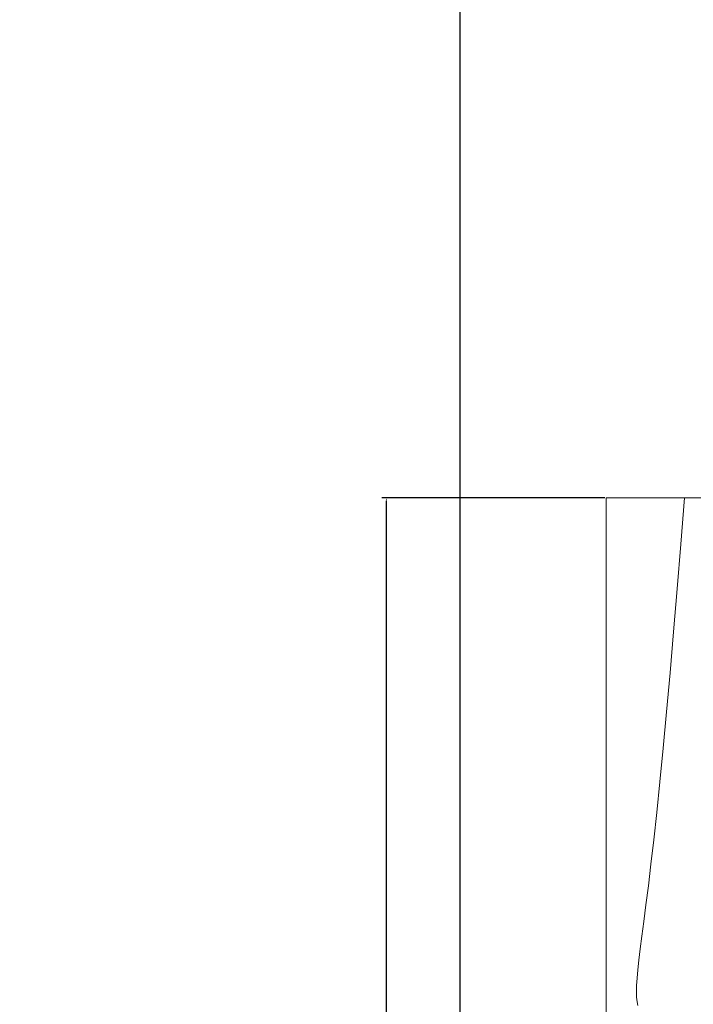
# Model space of a CAD drawing. Units: inches. Extents: x -301 to 715, y -607 to 364.
# Tile 108 of 141: x 16 to 43, y 107 to 147. Entities that reach past the tile are written whole.
import ezdxf

# ---------------------------------------------------------------- set-up
doc = ezdxf.new("R2010")
doc.units = ezdxf.units.IN
doc.header["$MEASUREMENT"] = 0
doc.layers.add('A-ANNO-DIMS', color=2, linetype='Continuous', lineweight=18)
doc.layers.add('A-FURN', color=8, linetype='Continuous', lineweight=18)
doc.styles.get("Standard").update_dxf_attribs({"font": 'arial.ttf'})
doc.dimstyles.get("Standard").update_dxf_attribs({"dimtxt": 0.18, "dimasz": 0.18, "dimexe": 0.18, "dimexo": 0.0625, "dimgap": 0.09, "dimtad": 0, "dimtih": 1, "dimtoh": 1, "dimdec": 1, "dimzin": 0, "dimdsep": 46, "dimlunit": 4, "dimtxsty": 'Standard', "dimcen": 0.09, "dimclrd": 3, "dimclre": 4, "dimclrt": 6, "dimadec": 0, "dimazin": 0, "dimtfac": 1, "dimtdec": 1, "dimtofl": 0, "dimtmove": 0, "dimatfit": 3, "dimfxl": 1, "dimtfill": 2, "dimtfillclr": 51, "dimtolj": 1, "dimtzin": 0, "dimarcsym": 0})

# ---------------------------------------------------------------- blocks, each defined once
blk = doc.blocks.new('Table - Rectangular Woodgrain 60 x 30 in.')
for p, q in [((60, 0), (0, 0)), ((60, -30), (60, 0))]:
    blk.add_line(p, q)
blk.add_lwpolyline([(39.2351, -1.2896), (39.3937, -1.2583), (39.5804, -1.2396), (39.8, -1.2333), (40.057, -1.2396), (40.3562, -1.2583), (40.7023, -1.2896), (41.1, -1.3333), (41.5547, -1.3895), (42.0755, -1.4573), (42.6721, -1.5361), (43.3542, -1.625), (44.1316, -1.7233), (45.014, -1.8302), (46.0114, -1.9449), (47.1333, -2.0667), (48.3862, -2.1947), (49.7625, -2.3281), (51.2513, -2.4663), (52.8416, -2.6083), (54.5226, -2.7535), (56.2833, -2.9011), (58.1127, -3.0501), (60, -3.2)])
blk = doc.blocks.new('*D49')
at = {"layer": 'A-ANNO-DIMS', "color": 0, "lineweight": -2, "transparency": 16777216}
for p, q in [((15.959, 193.182), (34.084, 193.182)), ((33.904, 188.182), (33.904, 93.304)), ((33.904, -4.818), (33.904, 90.061)), ((21.959, -9.818), (34.084, -9.818))]:
    blk.add_line(p, q, dxfattribs=at)
at = {"layer": 'A-ANNO-DIMS', "color": 0, "transparency": 16777216}
for points in [[(33.071, 188.182), (34.737, 188.182), (33.904, 193.182)], [(33.071, -4.818), (34.737, -4.818), (33.904, -9.818)]]:
    blk.add_solid(points, dxfattribs=at)
at = {"layer": 'Defpoints', "color": 0, "transparency": 16777216}
for p in [(15.897, 193.182), (33.904, 193.182), (21.897, -9.818)]:
    blk.add_point(p, dxfattribs=at)
at = {"layer": 'A-ANNO-DIMS', "color": 0, "transparency": 16777216, "insert": (33.904, 91.682), "char_height": 3, "attachment_point": 5, "bg_fill": 1, "box_fill_scale": 1.25, "bg_fill_color": 51, "bg_fill_transparency": 0}
blk.add_mtext('\\A1;16\'-11"', dxfattribs=at)
blk = doc.blocks.new('*D130')
at = {"layer": 'A-ANNO-DIMS', "color": 4, "lineweight": -2, "transparency": 16777216}
for p, q in [((39.835, 127.651), (30.717, 127.651)), ((39.835, 67.651), (30.717, 67.651))]:
    blk.add_line(p, q, dxfattribs=at)
at = {"layer": 'A-ANNO-DIMS', "color": 3, "lineweight": -2, "transparency": 16777216}
for p, q in [((30.897, 127.471), (30.897, 97.834)), ((30.897, 67.831), (30.897, 97.467))]:
    blk.add_line(p, q, dxfattribs=at)
at = {"layer": 'A-ANNO-DIMS', "color": 3, "transparency": 16777216}
for points in [[(30.867, 127.471), (30.927, 127.471), (30.897, 127.651)], [(30.867, 67.831), (30.927, 67.831), (30.897, 67.651)]]:
    blk.add_solid(points, dxfattribs=at)
at = {"layer": 'Defpoints', "color": 0, "transparency": 16777216}
for p in [(30.897, 127.651), (39.897, 127.651), (39.897, 67.651)]:
    blk.add_point(p, dxfattribs=at)
at = {"layer": 'A-ANNO-DIMS', "color": 6, "transparency": 16777216, "insert": (30.897, 97.651), "char_height": 0.18, "attachment_point": 5, "bg_fill": 1, "box_fill_scale": 1.25, "bg_fill_color": 51, "bg_fill_transparency": 0}
blk.add_mtext('\\A1;COFFEE TABLE 5\'-0"', dxfattribs=at)

msp = doc.modelspace()

# ---------------------------------------------------------------- block references
at = {"layer": 'A-FURN', "rotation": 90}
msp.add_blockref('Table - Rectangular Woodgrain 60 x 30 in.', (39.897, 67.651), dxfattribs=at)

# ---------------------------------------------------------------- dimensions: what is measured, and where the dimension line sits
at = {"layer": 'A-ANNO-DIMS'}
dim = msp.add_linear_dim(base=(33.904, 193.182), p1=(21.897, -9.818), p2=(15.897, 193.182), angle=90, dimstyle='Standard', override={"dimtxt": 3, "dimasz": 5, "dimclrd": 0, "dimclre": 0, "dimclrt": 0}, dxfattribs=at)
dim.commit()
dim.dimension.update_dxf_attribs({"geometry": '*D49', "text_midpoint": (33.904, 91.682)})
dim = msp.add_linear_dim(base=(30.897, 127.651), p1=(39.897, 67.651), p2=(39.897, 127.651), angle=90, text='COFFEE TABLE <>', dimstyle='Standard', override={"dimdec": 1, "dimlfac": 1, "dimrnd": 0, "dimzin": 1, "dimdsep": 46, "dimlunit": 4, "dimfrac": 2}, dxfattribs=at)
dim.commit()
dim.dimension.update_dxf_attribs({"geometry": '*D130', "text_midpoint": (30.897, 97.651)})

doc.saveas('drawing.dxf')
